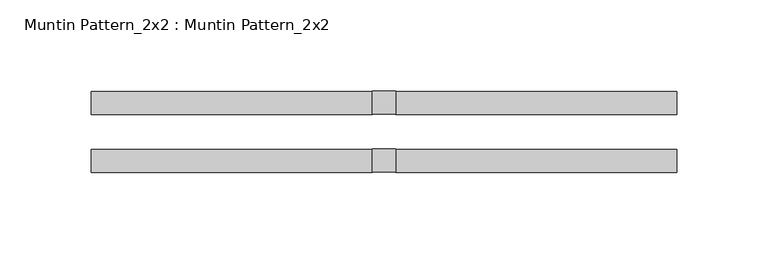
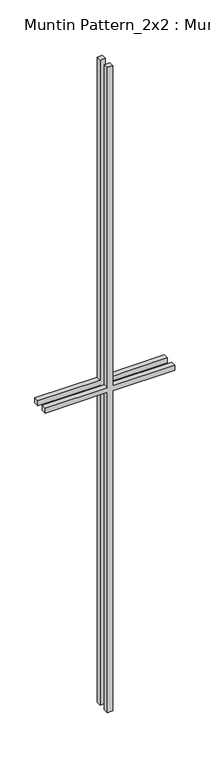
"""IFC4 building model written with IfcOpenShell, lengths in millimetres: proxy geometry, Muntin Pattern_2x2 : Muntin Pattern_2x2."""

from ifc_helpers import new_model, si_unit, frame, origin, place, context, project, spatial, polyline, outline, extrude, source, transform, mapped, element, save


def muntin_pattern_2x2_muntin_pattern_2x2_9767bead(model_context):
    return source(origin(), model_context, "Body", "SweptSolid", [
        extrude(outline(polyline([(850.9, -6.35), (850.9, -160.3375), (838.2, -160.3375), (838.2, -6.35), (0.0, -6.35), (0.0, 6.35), (838.2, 6.35), (838.2, 160.3375), (850.9, 160.3375), (850.9, 6.35), (1689.1, 6.35), (1689.1, -6.35), (850.9, -6.35)])), frame((0.0, -22.225, 0.0), z_axis=(0.0, 1.0, 0.0), x_axis=(0.0, 0.0, 1.0)), (0.0, 0.0, 1.0), 12.7),
        extrude(outline(polyline([(850.9, -6.35), (850.9, -160.3375), (838.2, -160.3375), (838.2, -6.35), (0.0, -6.35), (0.0, 6.35), (838.2, 6.35), (838.2, 160.3375), (850.9, 160.3375), (850.9, 6.35), (1689.1, 6.35), (1689.1, -6.35), (850.9, -6.35)])), frame((0.0, 9.525, 0.0), z_axis=(0.0, 1.0, 0.0), x_axis=(0.0, 0.0, 1.0)), (0.0, 0.0, 1.0), 12.7),
    ])


if __name__ == "__main__":
    model = new_model("IFC4")
    model_context = context("Model", 3, world=origin())
    ifc_project = project(units=[si_unit("LENGTHUNIT", "METRE", prefix="MILLI")], contexts=[model_context])
    site = spatial("IfcSite", under=ifc_project)
    building = spatial("IfcBuilding", under=site)
    placement = place(None, origin())
    muntin_pattern_2x2_muntin_pattern_2x2_shape = muntin_pattern_2x2_muntin_pattern_2x2_9767bead(model_context)
    element("IfcBuildingElementProxy", 1, Name="Muntin Pattern_2x2 : Muntin Pattern_2x2", ObjectType="Muntin Pattern_2x2 : Muntin Pattern_2x2", at=placement, inside=building, context=model_context, shape_type="MappedRepresentation", body=[
        mapped(muntin_pattern_2x2_muntin_pattern_2x2_shape, transform((0.0, 0.0, 0.0), x_axis=(1.0, 0.0, 0.0), y_axis=(0.0, 1.0, 0.0), z_axis=(0.0, 0.0, 1.0))),
    ])
    save(model, "model.ifc")

# Revit data of these elements
# Type "Muntin Pattern_2x2 : Muntin Pattern_2x2"
#   Width [instance default] = 4' - 0"
#   Thickness = 0' - 0 1/2"
#   Height [instance default] = 4' - 0"
#   Distance = 0' - 0 3/4"
#   Interior Material [instance default] = none
#   Exterior Material [instance default] = none
#   Default Elevation = 0
# Element 1 (IfcBuildingElementProxy, "Muntin Pattern_2x2 : Muntin Pattern_2x2")
#   Width = 1' - 0 5/8"
#   Height = 5' - 6 1/2"
#   Interior Material = Wood - Stained
#   Exterior Material = Clad - White
#   Materials on its faces: "Clad - White", "Wood - Stained"
# Materials
#   "Clad - White": class "Wood", colour RGB 242 242 238, transparency 0, Cost = 0
#   "Wood - Stained": class "Wood", colour RGB 224 178 126, transparency 0, Cost = 0
